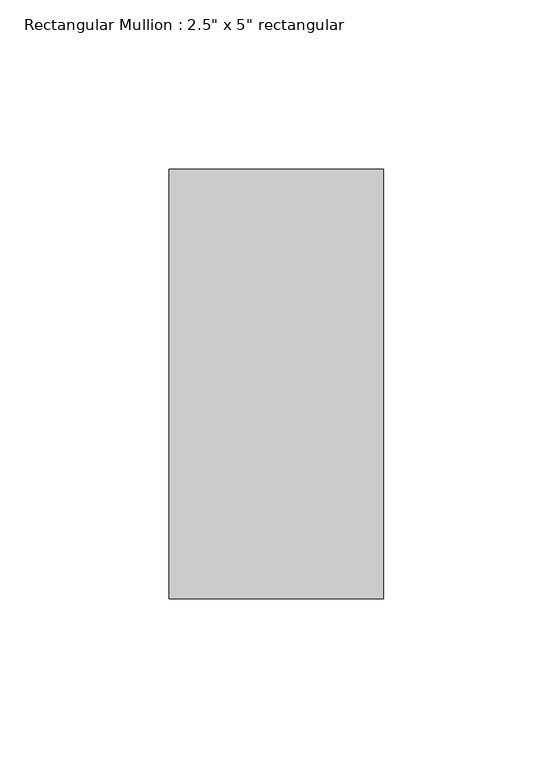
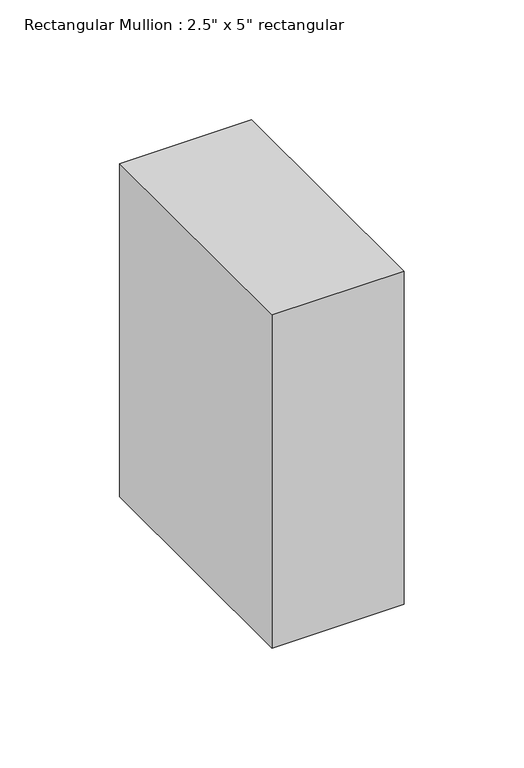
"""IFC4 building model written with IfcOpenShell, lengths in millimetres: member geometry."""

from ifc_helpers import new_model, si_unit, frame, origin, place, context, project, spatial, polyline, outline, extrude, source, transform, mapped, element, save


def member_2caf9219(model_context):
    return source(origin(), model_context, "Body", "SweptSolid", [
        extrude(outline(polyline([(0.0, 63.5), (0.0, -63.5), (-63.5, -63.5), (-63.5, 63.5), (0.0, 63.5)])), frame((0.0, 0.0, -169.4874164), z_axis=(0.0, 0.0, 1.0), x_axis=(1.0, 0.0, 0.0)), (0.0, 0.0, 1.0), 169.4874164),
    ])


if __name__ == "__main__":
    model = new_model("IFC4")
    model_context = context("Model", 3, world=origin())
    ifc_project = project(units=[si_unit("LENGTHUNIT", "METRE", prefix="MILLI")], contexts=[model_context])
    site = spatial("IfcSite", under=ifc_project)
    building = spatial("IfcBuilding", under=site)
    placement = place(None, origin())
    member_shape = member_2caf9219(model_context)
    element("IfcMember", 1, ObjectType="Rectangular Mullion : 2.5\" x 5\" rectangular", at=placement, inside=building, context=model_context, shape_type="MappedRepresentation", body=[
        mapped(member_shape, transform((0.0, 0.0, 0.0), x_axis=(1.0, 0.0, 0.0), y_axis=(0.0, 1.0, 0.0), z_axis=(0.0, 0.0, 1.0))),
    ])
    save(model, "model.ifc")

# Revit data of these elements
# Type "Rectangular Mullion : 2.5\" x 5\" rectangular"
#   built-in parameter 1007304 = 0.416667 (stored number, unit not read)
#   built-in parameter 1007301 = 0.104167 (stored number, unit not read)
#   built-in parameter 1007300 = 0.104167 (stored number, unit not read)
# Element 1 (IfcMember, "Rectangular Mullion : 2.5\" x 5\" rectangular")
#   Materials on its faces: "Aluminum"
# Materials
#   "Aluminum": class "Metal", colour RGB 247 247 247, transparency 0, Description = "Aluminum 6061", Cost = 0
